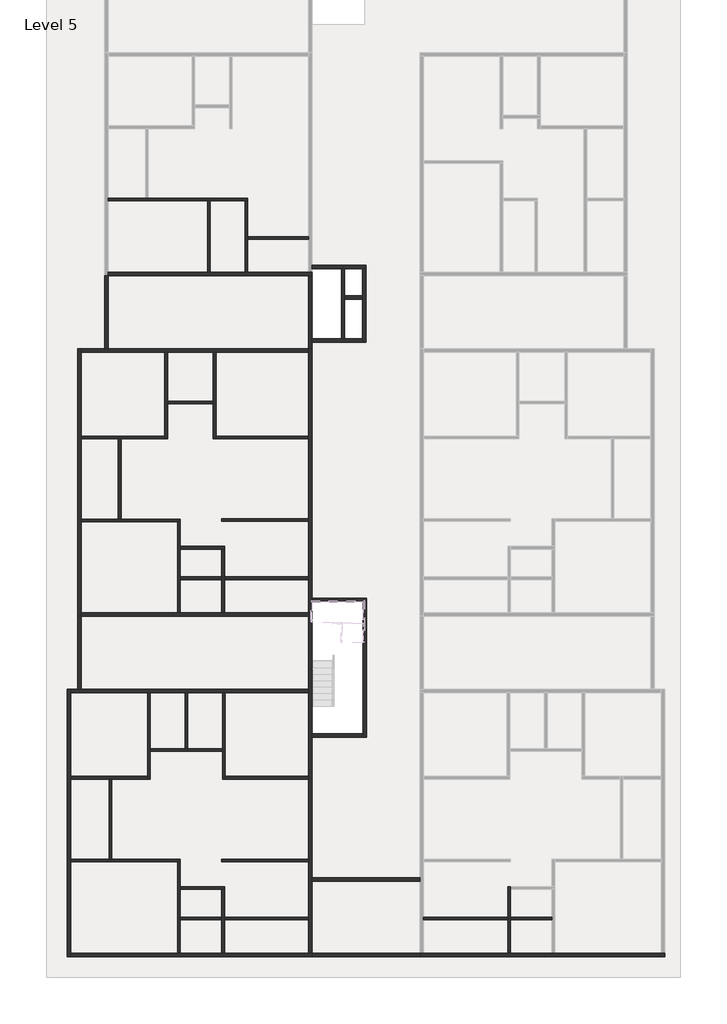
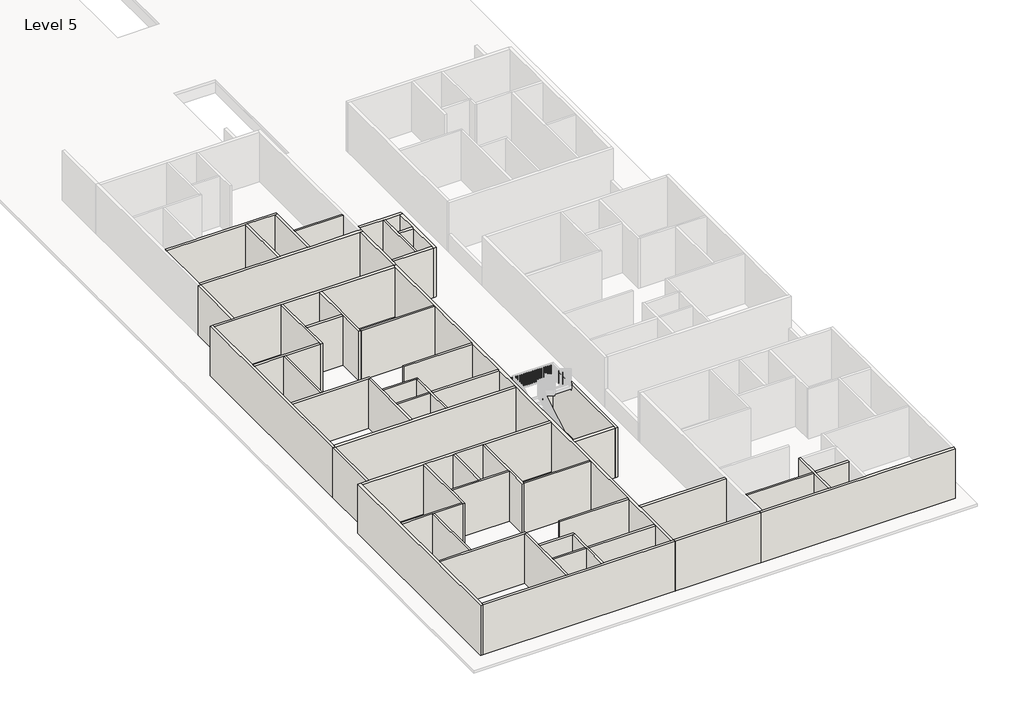
# One storey, part 1 of 8: 55 walls.
"""IFC4 building model written with IfcOpenShell, lengths in millimetres."""

from ifc_helpers import new_model, si_unit, frame, origin, place, context, project, spatial, polyline, outline, extrude, faceted_brep, element, save

model = new_model("IFC4")

# Units and contexts
model_context = context("Model", 3, world=origin())
ifc_project = project(units=[si_unit("LENGTHUNIT", "METRE", prefix="MILLI")], contexts=[model_context])

# Site, building, storey
site = spatial("IfcSite", under=ifc_project)
building = spatial("IfcBuilding", under=site)
storey = spatial("IfcBuildingStorey", under=building, Name="Level 5", Elevation=37426.6172466)

# Walls
placement = place(None, origin())
element("IfcWall", 1, ObjectType="4.5\"", at=placement, inside=storey, context=model_context, shape_type="Brep", body=[
    faceted_brep([(-12531.5544854, -1061.7344126, 37426.6172466), (-8188.1544854, -1061.7344126, 37426.6172466), (-8073.8544854, -1061.7344126, 37426.6172466), (-6549.8544854, -1061.7344126, 37426.6172466), (-6435.5544854, -1061.7344126, 37426.6172466), (-6435.5544854, -1061.7344126, 40474.6172466), (-6549.8544854, -1061.7344126, 40474.6172466), (-8073.8544854, -1061.7344126, 40474.6172466), (-8188.1544854, -1061.7344126, 40474.6172466), (-12531.5544854, -1061.7344126, 40474.6172466), (-12531.5544854, -947.4344126, 37426.6172466), (-12531.5544854, -947.4344126, 40474.6172466), (-10907.2415084, -947.4344126, 40474.6172466), (-10792.9415084, -947.4344126, 40474.6172466), (-6435.5544854, -947.4344126, 40474.6172466), (-6435.5544854, -947.4344126, 37426.6172466), (-10792.9415084, -947.4344126, 37426.6172466), (-10907.2415084, -947.4344126, 37426.6172466)], [[[0, 1, 2, 3, 4, 5, 6, 7, 8, 9]], [[10, 11, 12, 13, 14, 15, 16, 17]], [[4, 3, 2, 1, 0, 10, 17, 16, 15]], [[0, 9, 11, 10]], [[5, 4, 15, 14]], [[9, 8, 7, 6, 5, 14, 13, 12, 11]]]),
])
element("IfcWall", 2, ObjectType="4.5\"", at=placement, inside=storey, context=model_context, shape_type="Brep", body=[
    faceted_brep([(-6549.8544854, -1061.7344126, 37426.6172466), (-6549.8544854, -4185.9344126, 37426.6172466), (-6549.8544854, -4185.9344126, 40474.6172466), (-6549.8544854, -1061.7344126, 40474.6172466), (-6435.5544854, -1061.7344126, 37426.6172466), (-6435.5544854, -1061.7344126, 40474.6172466), (-6435.5544854, -2623.8344126, 40474.6172466), (-6435.5544854, -2738.1344126, 40474.6172466), (-6435.5544854, -4185.9344126, 40474.6172466), (-6435.5544854, -4185.9344126, 37426.6172466), (-6435.5544854, -2738.1344126, 37426.6172466), (-6435.5544854, -2623.8344126, 37426.6172466)], [[[0, 1, 2, 3]], [[4, 5, 6, 7, 8, 9, 10, 11]], [[1, 0, 4, 11, 10, 9]], [[0, 3, 5, 4]], [[2, 1, 9, 8]], [[3, 2, 8, 7, 6, 5]]]),
])
element("IfcWall", 3, ObjectType="4.5\"", at=placement, inside=storey, context=model_context, shape_type="SweptSolid", body=[
    extrude(outline(polyline([(-8188.1544854, -4185.9344126), (-8188.1544854, -1061.7344126), (-8073.8544854, -1061.7344126), (-8073.8544854, -4185.9344126), (-8188.1544854, -4185.9344126)])), frame((0.0, 0.0, 37426.6172466), z_axis=(0.0, 0.0, 1.0), x_axis=(1.0, 0.0, 0.0)), (0.0, 0.0, 1.0), 3048.0),
])
element("IfcWall", 4, ObjectType="4.5\"", at=placement, inside=storey, context=model_context, shape_type="SweptSolid", body=[
    extrude(outline(polyline([(-6435.5544854, -2623.8344126), (-3769.8415084, -2623.8344126), (-3769.8415084, -2738.1344126), (-6435.5544854, -2738.1344126), (-6435.5544854, -2623.8344126)])), frame((0.0, 0.0, 37426.6172466), z_axis=(0.0, 0.0, 1.0), x_axis=(1.0, 0.0, 0.0)), (0.0, 0.0, 1.0), 3048.0),
])
element("IfcWall", 5, ObjectType="4.5\"", at=placement, inside=storey, context=model_context, shape_type="Brep", body=[
    faceted_brep([(-10061.4044854, -7691.1344126, 37426.6172466), (-10061.4044854, -11348.7344126, 37426.6172466), (-10061.4044854, -11463.0344126, 37426.6172466), (-10061.4044854, -11463.0344126, 40474.6172466), (-10061.4044854, -11348.7344126, 40474.6172466), (-10061.4044854, -7691.1344126, 40474.6172466), (-9947.1044854, -7691.1344126, 37426.6172466), (-9947.1044854, -7691.1344126, 40474.6172466), (-9947.1044854, -9824.7344126, 40474.6172466), (-9947.1044854, -9939.0344126, 40474.6172466), (-9947.1044854, -11463.0344126, 40474.6172466), (-9947.1044854, -11463.0344126, 37426.6172466), (-9947.1044854, -9939.0344126, 37426.6172466), (-9947.1044854, -9824.7344126, 37426.6172466)], [[[0, 1, 2, 3, 4, 5]], [[6, 7, 8, 9, 10, 11, 12, 13]], [[2, 1, 0, 6, 13, 12, 11]], [[0, 5, 7, 6]], [[3, 2, 11, 10]], [[5, 4, 3, 10, 9, 8, 7]]]),
])
element("IfcWall", 6, ObjectType="4.5\"", at=placement, inside=storey, context=model_context, shape_type="Brep", body=[
    faceted_brep([(-10061.4044854, -11348.7344126, 37426.6172466), (-13719.0044854, -11348.7344126, 37426.6172466), (-13719.0044854, -11348.7344126, 40474.6172466), (-10061.4044854, -11348.7344126, 40474.6172466), (-10061.4044854, -11463.0344126, 37426.6172466), (-10061.4044854, -11463.0344126, 40474.6172466), (-11980.3915084, -11463.0344126, 40474.6172466), (-12094.6915084, -11463.0344126, 40474.6172466), (-13719.0044854, -11463.0344126, 40474.6172466), (-13719.0044854, -11463.0344126, 37426.6172466), (-12094.6915084, -11463.0344126, 37426.6172466), (-11980.3915084, -11463.0344126, 37426.6172466)], [[[0, 1, 2, 3]], [[4, 5, 6, 7, 8, 9, 10, 11]], [[1, 0, 4, 11, 10, 9]], [[0, 3, 5, 4]], [[2, 1, 9, 8]], [[3, 2, 8, 7, 6, 5]]]),
])
element("IfcWall", 7, ObjectType="4.5\"", at=placement, inside=storey, context=model_context, shape_type="SweptSolid", body=[
    extrude(outline(polyline([(-12094.6915084, -14968.2344126), (-12094.6915084, -11463.0344126), (-11980.3915084, -11463.0344126), (-11980.3915084, -14968.2344126), (-12094.6915084, -14968.2344126)])), frame((0.0, 0.0, 37426.6172466), z_axis=(0.0, 0.0, 1.0), x_axis=(1.0, 0.0, 0.0)), (0.0, 0.0, 1.0), 3048.0),
])
element("IfcWall", 8, ObjectType="4.5\"", at=placement, inside=storey, context=model_context, shape_type="Brep", body=[
    faceted_brep([(-13719.0044854, -15095.2344126, 37426.6172466), (-9510.2415084, -15095.2344126, 37426.6172466), (-9395.9415084, -15095.2344126, 37426.6172466), (-9395.9415084, -15095.2344126, 40474.6172466), (-9510.2415084, -15095.2344126, 40474.6172466), (-13719.0044854, -15095.2344126, 40474.6172466), (-13719.0044854, -14980.9344126, 37426.6172466), (-13719.0044854, -14980.9344126, 40474.6172466), (-9395.9415084, -14980.9344126, 40474.6172466), (-9395.9415084, -14980.9344126, 37426.6172466)], [[[0, 1, 2, 3, 4, 5]], [[6, 7, 8, 9]], [[2, 1, 0, 6, 9]], [[0, 5, 7, 6]], [[3, 2, 9, 8]], [[5, 4, 3, 8, 7]]]),
])
element("IfcWall", 9, ObjectType="4.5\"", at=placement, inside=storey, context=model_context, shape_type="Brep", body=[
    faceted_brep([(-9510.2415084, -15095.2344126, 37426.6172466), (-9510.2415084, -19070.3344126, 37426.6172466), (-9510.2415084, -19070.3344126, 40474.6172466), (-9510.2415084, -15095.2344126, 40474.6172466), (-9395.9415084, -15095.2344126, 37426.6172466), (-9395.9415084, -15095.2344126, 40474.6172466), (-9395.9415084, -16174.7344126, 40474.6172466), (-9395.9415084, -16289.0344126, 40474.6172466), (-9395.9415084, -17508.2344126, 40474.6172466), (-9395.9415084, -17622.5344126, 40474.6172466), (-9395.9415084, -19070.3344126, 40474.6172466), (-9395.9415084, -19070.3344126, 37426.6172466), (-9395.9415084, -17622.5344126, 37426.6172466), (-9395.9415084, -17508.2344126, 37426.6172466), (-9395.9415084, -16289.0344126, 37426.6172466), (-9395.9415084, -16174.7344126, 37426.6172466)], [[[0, 1, 2, 3]], [[4, 5, 6, 7, 8, 9, 10, 11, 12, 13, 14, 15]], [[1, 0, 4, 15, 14, 13, 12, 11]], [[0, 3, 5, 4]], [[2, 1, 11, 10]], [[3, 2, 10, 9, 8, 7, 6, 5]]]),
])
element("IfcWall", 10, ObjectType="4.5\"", at=placement, inside=storey, context=model_context, shape_type="Brep", body=[
    faceted_brep([(-9395.9415084, -16289.0344126, 37426.6172466), (-7567.1415084, -16289.0344126, 37426.6172466), (-7452.8415084, -16289.0344126, 37426.6172466), (-7452.8415084, -16289.0344126, 40474.6172466), (-7567.1415084, -16289.0344126, 40474.6172466), (-9395.9415084, -16289.0344126, 40474.6172466), (-9395.9415084, -16174.7344126, 37426.6172466), (-9395.9415084, -16174.7344126, 40474.6172466), (-7452.8415084, -16174.7344126, 40474.6172466), (-7452.8415084, -16174.7344126, 37426.6172466)], [[[0, 1, 2, 3, 4, 5]], [[6, 7, 8, 9]], [[2, 1, 0, 6, 9]], [[0, 5, 7, 6]], [[3, 2, 9, 8]], [[5, 4, 3, 8, 7]]]),
])
element("IfcWall", 11, ObjectType="4.5\"", at=placement, inside=storey, context=model_context, shape_type="Brep", body=[
    faceted_brep([(-7567.1415084, -16289.0344126, 37426.6172466), (-7567.1415084, -17508.2344126, 37426.6172466), (-7567.1415084, -17622.5344126, 37426.6172466), (-7567.1415084, -19070.3344126, 37426.6172466), (-7567.1415084, -19070.3344126, 40474.6172466), (-7567.1415084, -17622.5344126, 40474.6172466), (-7567.1415084, -17508.2344126, 40474.6172466), (-7567.1415084, -16289.0344126, 40474.6172466), (-7452.8415084, -16289.0344126, 37426.6172466), (-7452.8415084, -16289.0344126, 40474.6172466), (-7452.8415084, -17508.2344126, 40474.6172466), (-7452.8415084, -17622.5344126, 40474.6172466), (-7452.8415084, -19070.3344126, 40474.6172466), (-7452.8415084, -19070.3344126, 37426.6172466), (-7452.8415084, -17622.5344126, 37426.6172466), (-7452.8415084, -17508.2344126, 37426.6172466)], [[[0, 1, 2, 3, 4, 5, 6, 7]], [[8, 9, 10, 11, 12, 13, 14, 15]], [[3, 2, 1, 0, 8, 15, 14, 13]], [[0, 7, 9, 8]], [[4, 3, 13, 12]], [[7, 6, 5, 4, 12, 11, 10, 9]]]),
])
element("IfcWall", 12, ObjectType="4.5\"", at=placement, inside=storey, context=model_context, shape_type="SweptSolid", body=[
    extrude(outline(polyline([(-7567.1415084, -17622.5344126), (-9395.9415084, -17622.5344126), (-9395.9415084, -17508.2344126), (-7567.1415084, -17508.2344126), (-7567.1415084, -17622.5344126)])), frame((0.0, 0.0, 37426.6172466), z_axis=(0.0, 0.0, 1.0), x_axis=(1.0, 0.0, 0.0)), (0.0, 0.0, 1.0), 3048.0),
])
element("IfcWall", 13, ObjectType="4.5\"", at=placement, inside=storey, context=model_context, shape_type="SweptSolid", body=[
    extrude(outline(polyline([(-3769.8415084, -17622.5344126), (-7452.8415084, -17622.5344126), (-7452.8415084, -17508.2344126), (-3769.8415084, -17508.2344126), (-3769.8415084, -17622.5344126)])), frame((0.0, 0.0, 37426.6172466), z_axis=(0.0, 0.0, 1.0), x_axis=(1.0, 0.0, 0.0)), (0.0, 0.0, 1.0), 3048.0),
])
element("IfcWall", 14, ObjectType="4.5\"", at=placement, inside=storey, context=model_context, shape_type="SweptSolid", body=[
    extrude(outline(polyline([(-7567.1415084, -14968.2344126), (-3769.8415084, -14968.2344126), (-3769.8415084, -15082.5344126), (-7567.1415084, -15082.5344126), (-7567.1415084, -14968.2344126)])), frame((0.0, 0.0, 37426.6172466), z_axis=(0.0, 0.0, 1.0), x_axis=(1.0, 0.0, 0.0)), (0.0, 0.0, 1.0), 3048.0),
])
element("IfcWall", 15, ObjectType="4.5\"", at=placement, inside=storey, context=model_context, shape_type="SweptSolid", body=[
    extrude(outline(polyline([(-7940.5044854, -9939.0344126), (-9947.1044854, -9939.0344126), (-9947.1044854, -9824.7344126), (-7940.5044854, -9824.7344126), (-7940.5044854, -9939.0344126)])), frame((0.0, 0.0, 37426.6172466), z_axis=(0.0, 0.0, 1.0), x_axis=(1.0, 0.0, 0.0)), (0.0, 0.0, 1.0), 3048.0),
])
element("IfcWall", 16, ObjectType="4.5\"", at=placement, inside=storey, context=model_context, shape_type="Brep", body=[
    faceted_brep([(-7940.5044854, -7691.1344126, 37426.6172466), (-7940.5044854, -9824.7344126, 37426.6172466), (-7940.5044854, -9939.0344126, 37426.6172466), (-7940.5044854, -11463.0344126, 37426.6172466), (-7940.5044854, -11463.0344126, 40474.6172466), (-7940.5044854, -9939.0344126, 40474.6172466), (-7940.5044854, -9824.7344126, 40474.6172466), (-7940.5044854, -7691.1344126, 40474.6172466), (-7826.2044854, -7691.1344126, 37426.6172466), (-7826.2044854, -7691.1344126, 40474.6172466), (-7826.2044854, -11348.7344126, 40474.6172466), (-7826.2044854, -11463.0344126, 40474.6172466), (-7826.2044854, -11463.0344126, 37426.6172466), (-7826.2044854, -11348.7344126, 37426.6172466)], [[[0, 1, 2, 3, 4, 5, 6, 7]], [[8, 9, 10, 11, 12, 13]], [[3, 2, 1, 0, 8, 13, 12]], [[0, 7, 9, 8]], [[4, 3, 12, 11]], [[7, 6, 5, 4, 11, 10, 9]]]),
])
element("IfcWall", 17, ObjectType="4.5\"", at=placement, inside=storey, context=model_context, shape_type="SweptSolid", body=[
    extrude(outline(polyline([(-3769.8415084, -11463.0344126), (-7826.2044854, -11463.0344126), (-7826.2044854, -11348.7344126), (-3769.8415084, -11348.7344126), (-3769.8415084, -11463.0344126)])), frame((0.0, 0.0, 37426.6172466), z_axis=(0.0, 0.0, 1.0), x_axis=(1.0, 0.0, 0.0)), (0.0, 0.0, 1.0), 3048.0),
])
element("IfcWall", 18, ObjectType="4.5\"", at=placement, inside=storey, context=model_context, shape_type="Brep", body=[
    faceted_brep([(-10818.3415084, -22575.5344126, 37426.6172466), (-10818.3415084, -26233.1344126, 37426.6172466), (-10818.3415084, -26347.4344126, 37426.6172466), (-10818.3415084, -26347.4344126, 40474.6172466), (-10818.3415084, -26233.1344126, 40474.6172466), (-10818.3415084, -22575.5344126, 40474.6172466), (-10704.0415084, -22575.5344126, 37426.6172466), (-10704.0415084, -22575.5344126, 40474.6172466), (-10704.0415084, -25013.9344126, 40474.6172466), (-10704.0415084, -25128.2344126, 40474.6172466), (-10704.0415084, -26347.4344126, 40474.6172466), (-10704.0415084, -26347.4344126, 37426.6172466), (-10704.0415084, -25128.2344126, 37426.6172466), (-10704.0415084, -25013.9344126, 37426.6172466)], [[[0, 1, 2, 3, 4, 5]], [[6, 7, 8, 9, 10, 11, 12, 13]], [[2, 1, 0, 6, 13, 12, 11]], [[0, 5, 7, 6]], [[3, 2, 11, 10]], [[5, 4, 3, 10, 9, 8, 7]]]),
])
element("IfcWall", 19, ObjectType="4.5\"", at=placement, inside=storey, context=model_context, shape_type="Brep", body=[
    faceted_brep([(-10818.3415084, -26233.1344126, 37426.6172466), (-14171.1415084, -26233.1344126, 37426.6172466), (-14171.1415084, -26233.1344126, 40474.6172466), (-10818.3415084, -26233.1344126, 40474.6172466), (-10818.3415084, -26347.4344126, 37426.6172466), (-10818.3415084, -26347.4344126, 40474.6172466), (-12380.4415084, -26347.4344126, 40474.6172466), (-12494.7415084, -26347.4344126, 40474.6172466), (-14171.1415084, -26347.4344126, 40474.6172466), (-14171.1415084, -26347.4344126, 37426.6172466), (-12494.7415084, -26347.4344126, 37426.6172466), (-12380.4415084, -26347.4344126, 37426.6172466)], [[[0, 1, 2, 3]], [[4, 5, 6, 7, 8, 9, 10, 11]], [[1, 0, 4, 11, 10, 9]], [[0, 3, 5, 4]], [[2, 1, 9, 8]], [[3, 2, 8, 7, 6, 5]]]),
])
element("IfcWall", 20, ObjectType="4.5\"", at=placement, inside=storey, context=model_context, shape_type="SweptSolid", body=[
    extrude(outline(polyline([(-9180.0415084, -25013.9344126), (-9180.0415084, -22575.5344126), (-9065.7415084, -22575.5344126), (-9065.7415084, -25013.9344126), (-9180.0415084, -25013.9344126)])), frame((0.0, 0.0, 37426.6172466), z_axis=(0.0, 0.0, 1.0), x_axis=(1.0, 0.0, 0.0)), (0.0, 0.0, 1.0), 3048.0),
])
element("IfcWall", 21, ObjectType="4.5\"", at=placement, inside=storey, context=model_context, shape_type="Brep", body=[
    faceted_brep([(-10704.0415084, -25128.2344126, 37426.6172466), (-7541.7415084, -25128.2344126, 37426.6172466), (-7541.7415084, -25128.2344126, 40474.6172466), (-10704.0415084, -25128.2344126, 40474.6172466), (-10704.0415084, -25013.9344126, 37426.6172466), (-10704.0415084, -25013.9344126, 40474.6172466), (-9180.0415084, -25013.9344126, 40474.6172466), (-9065.7415084, -25013.9344126, 40474.6172466), (-7541.7415084, -25013.9344126, 40474.6172466), (-7541.7415084, -25013.9344126, 37426.6172466), (-9065.7415084, -25013.9344126, 37426.6172466), (-9180.0415084, -25013.9344126, 37426.6172466)], [[[0, 1, 2, 3]], [[4, 5, 6, 7, 8, 9, 10, 11]], [[1, 0, 4, 11, 10, 9]], [[0, 3, 5, 4]], [[2, 1, 9, 8]], [[3, 2, 8, 7, 6, 5]]]),
])
element("IfcWall", 22, ObjectType="4.5\"", at=placement, inside=storey, context=model_context, shape_type="Brep", body=[
    faceted_brep([(-7541.7415084, -22575.5344126, 37426.6172466), (-7541.7415084, -25013.9344126, 37426.6172466), (-7541.7415084, -25128.2344126, 37426.6172466), (-7541.7415084, -26347.4344126, 37426.6172466), (-7541.7415084, -26347.4344126, 40474.6172466), (-7541.7415084, -25128.2344126, 40474.6172466), (-7541.7415084, -25013.9344126, 40474.6172466), (-7541.7415084, -22575.5344126, 40474.6172466), (-7427.4415084, -22575.5344126, 37426.6172466), (-7427.4415084, -22575.5344126, 40474.6172466), (-7427.4415084, -26233.1344126, 40474.6172466), (-7427.4415084, -26347.4344126, 40474.6172466), (-7427.4415084, -26347.4344126, 37426.6172466), (-7427.4415084, -26233.1344126, 37426.6172466)], [[[0, 1, 2, 3, 4, 5, 6, 7]], [[8, 9, 10, 11, 12, 13]], [[3, 2, 1, 0, 8, 13, 12]], [[0, 7, 9, 8]], [[4, 3, 12, 11]], [[7, 6, 5, 4, 11, 10, 9]]]),
])
element("IfcWall", 23, ObjectType="4.5\"", at=placement, inside=storey, context=model_context, shape_type="SweptSolid", body=[
    extrude(outline(polyline([(-3769.8415084, -26347.4344126), (-7427.4415084, -26347.4344126), (-7427.4415084, -26233.1344126), (-3769.8415084, -26233.1344126), (-3769.8415084, -26347.4344126)])), frame((0.0, 0.0, 37426.6172466), z_axis=(0.0, 0.0, 1.0), x_axis=(1.0, 0.0, 0.0)), (0.0, 0.0, 1.0), 3048.0),
])
element("IfcWall", 24, ObjectType="4.5\"", at=placement, inside=storey, context=model_context, shape_type="SweptSolid", body=[
    extrude(outline(polyline([(-12494.7415084, -29852.6344126), (-12494.7415084, -26347.4344126), (-12380.4415084, -26347.4344126), (-12380.4415084, -29852.6344126), (-12494.7415084, -29852.6344126)])), frame((0.0, 0.0, 37426.6172466), z_axis=(0.0, 0.0, 1.0), x_axis=(1.0, 0.0, 0.0)), (0.0, 0.0, 1.0), 3048.0),
])
element("IfcWall", 25, ObjectType="4.5\"", at=placement, inside=storey, context=model_context, shape_type="Brep", body=[
    faceted_brep([(-14171.1415084, -29966.9344126, 37426.6172466), (-9510.2415084, -29966.9344126, 37426.6172466), (-9395.9415084, -29966.9344126, 37426.6172466), (-9395.9415084, -29966.9344126, 40474.6172466), (-9510.2415084, -29966.9344126, 40474.6172466), (-14171.1415084, -29966.9344126, 40474.6172466), (-14171.1415084, -29852.6344126, 37426.6172466), (-14171.1415084, -29852.6344126, 40474.6172466), (-12494.7415084, -29852.6344126, 40474.6172466), (-12380.4415084, -29852.6344126, 40474.6172466), (-9395.9415084, -29852.6344126, 40474.6172466), (-9395.9415084, -29852.6344126, 37426.6172466), (-12380.4415084, -29852.6344126, 37426.6172466), (-12494.7415084, -29852.6344126, 37426.6172466)], [[[0, 1, 2, 3, 4, 5]], [[6, 7, 8, 9, 10, 11, 12, 13]], [[2, 1, 0, 6, 13, 12, 11]], [[0, 5, 7, 6]], [[3, 2, 11, 10]], [[5, 4, 3, 10, 9, 8, 7]]]),
])
element("IfcWall", 26, ObjectType="4.5\"", at=placement, inside=storey, context=model_context, shape_type="Brep", body=[
    faceted_brep([(-9510.2415084, -29966.9344126, 37426.6172466), (-9510.2415084, -33954.7344126, 37426.6172466), (-9510.2415084, -33954.7344126, 40474.6172466), (-9510.2415084, -29966.9344126, 40474.6172466), (-9395.9415084, -29966.9344126, 37426.6172466), (-9395.9415084, -29966.9344126, 40474.6172466), (-9395.9415084, -31059.1344126, 40474.6172466), (-9395.9415084, -31173.4344126, 40474.6172466), (-9395.9415084, -32392.6344126, 40474.6172466), (-9395.9415084, -32506.9344126, 40474.6172466), (-9395.9415084, -33954.7344126, 40474.6172466), (-9395.9415084, -33954.7344126, 37426.6172466), (-9395.9415084, -32506.9344126, 37426.6172466), (-9395.9415084, -32392.6344126, 37426.6172466), (-9395.9415084, -31173.4344126, 37426.6172466), (-9395.9415084, -31059.1344126, 37426.6172466)], [[[0, 1, 2, 3]], [[4, 5, 6, 7, 8, 9, 10, 11, 12, 13, 14, 15]], [[1, 0, 4, 15, 14, 13, 12, 11]], [[0, 3, 5, 4]], [[2, 1, 11, 10]], [[3, 2, 10, 9, 8, 7, 6, 5]]]),
])
element("IfcWall", 27, ObjectType="4.5\"", at=placement, inside=storey, context=model_context, shape_type="Brep", body=[
    faceted_brep([(-9395.9415084, -31173.4344126, 37426.6172466), (-7567.1415084, -31173.4344126, 37426.6172466), (-7452.8415084, -31173.4344126, 37426.6172466), (-7452.8415084, -31173.4344126, 40474.6172466), (-7567.1415084, -31173.4344126, 40474.6172466), (-9395.9415084, -31173.4344126, 40474.6172466), (-9395.9415084, -31059.1344126, 37426.6172466), (-9395.9415084, -31059.1344126, 40474.6172466), (-7452.8415084, -31059.1344126, 40474.6172466), (-7452.8415084, -31059.1344126, 37426.6172466)], [[[0, 1, 2, 3, 4, 5]], [[6, 7, 8, 9]], [[2, 1, 0, 6, 9]], [[0, 5, 7, 6]], [[3, 2, 9, 8]], [[5, 4, 3, 8, 7]]]),
])
element("IfcWall", 28, ObjectType="4.5\"", at=placement, inside=storey, context=model_context, shape_type="Brep", body=[
    faceted_brep([(-7567.1415084, -31173.4344126, 37426.6172466), (-7567.1415084, -32392.6344126, 37426.6172466), (-7567.1415084, -32506.9344126, 37426.6172466), (-7567.1415084, -33954.7344126, 37426.6172466), (-7567.1415084, -33954.7344126, 40474.6172466), (-7567.1415084, -32506.9344126, 40474.6172466), (-7567.1415084, -32392.6344126, 40474.6172466), (-7567.1415084, -31173.4344126, 40474.6172466), (-7452.8415084, -31173.4344126, 37426.6172466), (-7452.8415084, -31173.4344126, 40474.6172466), (-7452.8415084, -32392.6344126, 40474.6172466), (-7452.8415084, -32506.9344126, 40474.6172466), (-7452.8415084, -33954.7344126, 40474.6172466), (-7452.8415084, -33954.7344126, 37426.6172466), (-7452.8415084, -32506.9344126, 37426.6172466), (-7452.8415084, -32392.6344126, 37426.6172466)], [[[0, 1, 2, 3, 4, 5, 6, 7]], [[8, 9, 10, 11, 12, 13, 14, 15]], [[3, 2, 1, 0, 8, 15, 14, 13]], [[0, 7, 9, 8]], [[4, 3, 13, 12]], [[7, 6, 5, 4, 12, 11, 10, 9]]]),
])
element("IfcWall", 29, ObjectType="4.5\"", at=placement, inside=storey, context=model_context, shape_type="SweptSolid", body=[
    extrude(outline(polyline([(-3769.8415084, -32392.6344126), (-3769.8415084, -32506.9344126), (-7452.8415084, -32506.9344126), (-7452.8415084, -32392.6344126), (-3769.8415084, -32392.6344126)])), frame((0.0, 0.0, 37426.6172466), z_axis=(0.0, 0.0, 1.0), x_axis=(1.0, 0.0, 0.0)), (0.0, 0.0, 1.0), 3048.0),
    extrude(outline(polyline([(-9395.9415084, -32506.9344126), (-9395.9415084, -32392.6344126), (-7567.1415084, -32392.6344126), (-7567.1415084, -32506.9344126), (-9395.9415084, -32506.9344126)])), frame((0.0, 0.0, 37426.6172466), z_axis=(0.0, 0.0, 1.0), x_axis=(1.0, 0.0, 0.0)), (0.0, 0.0, 1.0), 3048.0),
])
element("IfcWall", 30, ObjectType="4.5\"", at=placement, inside=storey, context=model_context, shape_type="SweptSolid", body=[
    extrude(outline(polyline([(-7567.1415084, -29852.6344126), (-3769.8415084, -29852.6344126), (-3769.8415084, -29966.9344126), (-7567.1415084, -29966.9344126), (-7567.1415084, -29852.6344126)])), frame((0.0, 0.0, 37426.6172466), z_axis=(0.0, 0.0, 1.0), x_axis=(1.0, 0.0, 0.0)), (0.0, 0.0, 1.0), 3048.0),
])
element("IfcWall", 31, ObjectType="4.5\"", at=placement, inside=storey, context=model_context, shape_type="SweptSolid", body=[
    extrude(outline(polyline([(4942.3584916, -32506.9344126), (1259.3584916, -32506.9344126), (1259.3584916, -32392.6344126), (4942.3584916, -32392.6344126), (4942.3584916, -32506.9344126)])), frame((0.0, 0.0, 37426.6172466), z_axis=(0.0, 0.0, 1.0), x_axis=(1.0, 0.0, 0.0)), (0.0, 0.0, 1.0), 3048.0),
])
element("IfcWall", 32, ObjectType="4.5\"", at=placement, inside=storey, context=model_context, shape_type="Brep", body=[
    faceted_brep([(4942.3584916, -31059.1344126, 37426.6172466), (4942.3584916, -32392.6344126, 37426.6172466), (4942.3584916, -32506.9344126, 37426.6172466), (4942.3584916, -33954.7344126, 37426.6172466), (4942.3584916, -33954.7344126, 40474.6172466), (4942.3584916, -32506.9344126, 40474.6172466), (4942.3584916, -32392.6344126, 40474.6172466), (4942.3584916, -31059.1344126, 40474.6172466), (5056.6584916, -31059.1344126, 37426.6172466), (5056.6584916, -31059.1344126, 40474.6172466), (5056.6584916, -31173.4344126, 40474.6172466), (5056.6584916, -32392.6344126, 40474.6172466), (5056.6584916, -32506.9344126, 40474.6172466), (5056.6584916, -33954.7344126, 40474.6172466), (5056.6584916, -33954.7344126, 37426.6172466), (5056.6584916, -32506.9344126, 37426.6172466), (5056.6584916, -32392.6344126, 37426.6172466), (5056.6584916, -31173.4344126, 37426.6172466)], [[[0, 1, 2, 3, 4, 5, 6, 7]], [[8, 9, 10, 11, 12, 13, 14, 15, 16, 17]], [[3, 2, 1, 0, 8, 17, 16, 15, 14]], [[4, 3, 14, 13]], [[0, 7, 9, 8]], [[7, 6, 5, 4, 13, 12, 11, 10, 9]]]),
])
element("IfcWall", 33, ObjectType="4.5\"", at=placement, inside=storey, context=model_context, shape_type="SweptSolid", body=[
    extrude(outline(polyline([(6885.4584916, -32506.9344126), (5056.6584916, -32506.9344126), (5056.6584916, -32392.6344126), (6885.4584916, -32392.6344126), (6885.4584916, -32506.9344126)])), frame((0.0, 0.0, 37426.6172466), z_axis=(0.0, 0.0, 1.0), x_axis=(1.0, 0.0, 0.0)), (0.0, 0.0, 1.0), 3048.0),
])
element("IfcWall", 34, ObjectType="4.5\"", at=placement, inside=storey, context=model_context, shape_type="Brep", body=[
    faceted_brep([(-2207.6738684, -7082.6751812, 37426.6172466), (-2207.6738684, -5366.3479894, 37426.6172466), (-2207.6738684, -5213.9479894, 37426.6172466), (-2207.6738684, -4034.6751812, 37426.6172466), (-2207.6738684, -4034.6751812, 40474.6172466), (-2207.6738684, -5213.9479894, 40474.6172466), (-2207.6738684, -5366.3479894, 40474.6172466), (-2207.6738684, -7082.6751812, 40474.6172466), (-2321.9738684, -7082.6751812, 37426.6172466), (-2321.9738684, -7082.6751812, 40474.6172466), (-2321.9738684, -4034.6751812, 40474.6172466), (-2321.9738684, -4034.6751812, 37426.6172466)], [[[0, 1, 2, 3, 4, 5, 6, 7]], [[8, 9, 10, 11]], [[3, 2, 1, 0, 8, 11]], [[7, 6, 5, 4, 10, 9]], [[4, 3, 11, 10]], [[0, 7, 9, 8]]]),
])
element("IfcWall", 35, ObjectType="6\"", at=placement, inside=storey, context=model_context, shape_type="Brep", body=[
    faceted_brep([(-12531.5544854, -4338.3344126, 37426.6172466), (-3769.8415084, -4338.3344126, 37426.6172466), (-3617.4415084, -4338.3344126, 37426.6172466), (-3617.4415084, -4338.3344126, 40474.6172466), (-3769.8415084, -4338.3344126, 40474.6172466), (-12531.5544854, -4338.3344126, 40474.6172466), (-12531.5544854, -4185.9344126, 37426.6172466), (-12531.5544854, -4185.9344126, 40474.6172466), (-8188.1544854, -4185.9344126, 40474.6172466), (-8073.8544854, -4185.9344126, 40474.6172466), (-6549.8544854, -4185.9344126, 40474.6172466), (-6435.5544854, -4185.9344126, 40474.6172466), (-3769.8415084, -4185.9344126, 40474.6172466), (-3617.4415084, -4185.9344126, 40474.6172466), (-3617.4415084, -4185.9344126, 37426.6172466), (-3769.8415084, -4185.9344126, 37426.6172466), (-6435.5544854, -4185.9344126, 37426.6172466), (-6549.8544854, -4185.9344126, 37426.6172466), (-8073.8544854, -4185.9344126, 37426.6172466), (-8188.1544854, -4185.9344126, 37426.6172466)], [[[0, 1, 2, 3, 4, 5]], [[6, 7, 8, 9, 10, 11, 12, 13, 14, 15, 16, 17, 18, 19]], [[2, 1, 0, 6, 19, 18, 17, 16, 15, 14]], [[0, 5, 7, 6]], [[3, 2, 14, 13]], [[5, 4, 3, 13, 12, 11, 10, 9, 8, 7]]]),
])
element("IfcWall", 36, ObjectType="6\"", at=placement, inside=storey, context=model_context, shape_type="Brep", body=[
    faceted_brep([(-13871.4044854, -7538.7344126, 37426.6172466), (-13871.4044854, -19222.7344126, 37426.6172466), (-13871.4044854, -19222.7344126, 40474.6172466), (-13871.4044854, -7538.7344126, 40474.6172466), (-13719.0044854, -7538.7344126, 37426.6172466), (-13719.0044854, -7538.7344126, 40474.6172466), (-13719.0044854, -7691.1344126, 40474.6172466), (-13719.0044854, -11348.7344126, 40474.6172466), (-13719.0044854, -11463.0344126, 40474.6172466), (-13719.0044854, -14980.9344126, 40474.6172466), (-13719.0044854, -15095.2344126, 40474.6172466), (-13719.0044854, -19070.3344126, 40474.6172466), (-13719.0044854, -19222.7344126, 40474.6172466), (-13719.0044854, -19222.7344126, 37426.6172466), (-13719.0044854, -19070.3344126, 37426.6172466), (-13719.0044854, -15095.2344126, 37426.6172466), (-13719.0044854, -14980.9344126, 37426.6172466), (-13719.0044854, -11463.0344126, 37426.6172466), (-13719.0044854, -11348.7344126, 37426.6172466), (-13719.0044854, -7691.1344126, 37426.6172466)], [[[0, 1, 2, 3]], [[4, 5, 6, 7, 8, 9, 10, 11, 12, 13, 14, 15, 16, 17, 18, 19]], [[1, 0, 4, 19, 18, 17, 16, 15, 14, 13]], [[2, 1, 13, 12]], [[0, 3, 5, 4]], [[3, 2, 12, 11, 10, 9, 8, 7, 6, 5]]]),
])
element("IfcWall", 37, ObjectType="6\"", at=placement, inside=storey, context=model_context, shape_type="Brep", body=[
    faceted_brep([(-13719.0044854, -19222.7344126, 37426.6172466), (-3769.8415084, -19222.7344126, 37426.6172466), (-3769.8415084, -19222.7344126, 40474.6172466), (-13719.0044854, -19222.7344126, 40474.6172466), (-13719.0044854, -19070.3344126, 37426.6172466), (-13719.0044854, -19070.3344126, 40474.6172466), (-9510.2415084, -19070.3344126, 40474.6172466), (-9395.9415084, -19070.3344126, 40474.6172466), (-7567.1415084, -19070.3344126, 40474.6172466), (-7452.8415084, -19070.3344126, 40474.6172466), (-3769.8415084, -19070.3344126, 40474.6172466), (-3769.8415084, -19070.3344126, 37426.6172466), (-7452.8415084, -19070.3344126, 37426.6172466), (-7567.1415084, -19070.3344126, 37426.6172466), (-9395.9415084, -19070.3344126, 37426.6172466), (-9510.2415084, -19070.3344126, 37426.6172466)], [[[0, 1, 2, 3]], [[4, 5, 6, 7, 8, 9, 10, 11, 12, 13, 14, 15]], [[1, 0, 4, 15, 14, 13, 12, 11]], [[0, 3, 5, 4]], [[2, 1, 11, 10]], [[3, 2, 10, 9, 8, 7, 6, 5]]]),
])
element("IfcWall", 38, ObjectType="6\"", at=placement, inside=storey, context=model_context, shape_type="Brep", body=[
    faceted_brep([(-3617.4415084, -33954.7344126, 37426.6172466), (-3617.4415084, -30820.9325185, 37426.6172466), (-3617.4415084, -30668.5325185, 37426.6172466), (-3617.4415084, -24525.9851539, 37426.6172466), (-3617.4415084, -24373.5851539, 37426.6172466), (-3617.4415084, -18582.3851539, 37426.6172466), (-3617.4415084, -18429.9851539, 37426.6172466), (-3617.4415084, -7538.7344126, 37426.6172466), (-3617.4415084, -7538.7344126, 40474.6172466), (-3617.4415084, -18429.9851539, 40474.6172466), (-3617.4415084, -18582.3851539, 40474.6172466), (-3617.4415084, -24373.5851539, 40474.6172466), (-3617.4415084, -24525.9851539, 40474.6172466), (-3617.4415084, -30668.5325185, 40474.6172466), (-3617.4415084, -30820.9325185, 40474.6172466), (-3617.4415084, -33954.7344126, 40474.6172466), (-3769.8415084, -33954.7344126, 37426.6172466), (-3769.8415084, -33954.7344126, 40474.6172466), (-3769.8415084, -32506.9344126, 40474.6172466), (-3769.8415084, -32392.6344126, 40474.6172466), (-3769.8415084, -29966.9344126, 40474.6172466), (-3769.8415084, -29852.6344126, 40474.6172466), (-3769.8415084, -26347.4344126, 40474.6172466), (-3769.8415084, -26233.1344126, 40474.6172466), (-3769.8415084, -22575.5344126, 40474.6172466), (-3769.8415084, -22423.1344126, 40474.6172466), (-3769.8415084, -19222.7344126, 40474.6172466), (-3769.8415084, -19070.3344126, 40474.6172466), (-3769.8415084, -17622.5344126, 40474.6172466), (-3769.8415084, -17508.2344126, 40474.6172466), (-3769.8415084, -15082.5344126, 40474.6172466), (-3769.8415084, -14968.2344126, 40474.6172466), (-3769.8415084, -11463.0344126, 40474.6172466), (-3769.8415084, -11348.7344126, 40474.6172466), (-3769.8415084, -7691.1344126, 40474.6172466), (-3769.8415084, -7538.7344126, 40474.6172466), (-3769.8415084, -7538.7344126, 37426.6172466), (-3769.8415084, -7691.1344126, 37426.6172466), (-3769.8415084, -11348.7344126, 37426.6172466), (-3769.8415084, -11463.0344126, 37426.6172466), (-3769.8415084, -14968.2344126, 37426.6172466), (-3769.8415084, -15082.5344126, 37426.6172466), (-3769.8415084, -17508.2344126, 37426.6172466), (-3769.8415084, -17622.5344126, 37426.6172466), (-3769.8415084, -19070.3344126, 37426.6172466), (-3769.8415084, -19222.7344126, 37426.6172466), (-3769.8415084, -22423.1344126, 37426.6172466), (-3769.8415084, -22575.5344126, 37426.6172466), (-3769.8415084, -26233.1344126, 37426.6172466), (-3769.8415084, -26347.4344126, 37426.6172466), (-3769.8415084, -29852.6344126, 37426.6172466), (-3769.8415084, -29966.9344126, 37426.6172466), (-3769.8415084, -32392.6344126, 37426.6172466), (-3769.8415084, -32506.9344126, 37426.6172466)], [[[0, 1, 2, 3, 4, 5, 6, 7, 8, 9, 10, 11, 12, 13, 14, 15]], [[16, 17, 18, 19, 20, 21, 22, 23, 24, 25, 26, 27, 28, 29, 30, 31, 32, 33, 34, 35, 36, 37, 38, 39, 40, 41, 42, 43, 44, 45, 46, 47, 48, 49, 50, 51, 52, 53]], [[7, 6, 5, 4, 3, 2, 1, 0, 16, 53, 52, 51, 50, 49, 48, 47, 46, 45, 44, 43, 42, 41, 40, 39, 38, 37, 36]], [[8, 7, 36, 35]], [[0, 15, 17, 16]], [[15, 14, 13, 12, 11, 10, 9, 8, 35, 34, 33, 32, 31, 30, 29, 28, 27, 26, 25, 24, 23, 22, 21, 20, 19, 18, 17]]]),
])
element("IfcWall", 39, ObjectType="6\"", at=placement, inside=storey, context=model_context, shape_type="Brep", body=[
    faceted_brep([(-3769.8415084, -7538.7344126, 37426.6172466), (-12531.5544854, -7538.7344126, 37426.6172466), (-12683.9544854, -7538.7344126, 37426.6172466), (-13719.0044854, -7538.7344126, 37426.6172466), (-13719.0044854, -7538.7344126, 40474.6172466), (-12683.9544854, -7538.7344126, 40474.6172466), (-12531.5544854, -7538.7344126, 40474.6172466), (-3769.8415084, -7538.7344126, 40474.6172466), (-3769.8415084, -7691.1344126, 37426.6172466), (-3769.8415084, -7691.1344126, 40474.6172466), (-7826.2044854, -7691.1344126, 40474.6172466), (-7940.5044854, -7691.1344126, 40474.6172466), (-9947.1044854, -7691.1344126, 40474.6172466), (-10061.4044854, -7691.1344126, 40474.6172466), (-13719.0044854, -7691.1344126, 40474.6172466), (-13719.0044854, -7691.1344126, 37426.6172466), (-10061.4044854, -7691.1344126, 37426.6172466), (-9947.1044854, -7691.1344126, 37426.6172466), (-7940.5044854, -7691.1344126, 37426.6172466), (-7826.2044854, -7691.1344126, 37426.6172466)], [[[0, 1, 2, 3, 4, 5, 6, 7]], [[8, 9, 10, 11, 12, 13, 14, 15, 16, 17, 18, 19]], [[3, 2, 1, 0, 8, 19, 18, 17, 16, 15]], [[0, 7, 9, 8]], [[4, 3, 15, 14]], [[7, 6, 5, 4, 14, 13, 12, 11, 10, 9]]]),
])
element("IfcWall", 40, ObjectType="6\"", at=placement, inside=storey, context=model_context, shape_type="Brep", body=[
    faceted_brep([(-14323.5415084, -22423.1344126, 37426.6172466), (-14323.5415084, -34107.1344126, 37426.6172466), (-14323.5415084, -34107.1344126, 40474.6172466), (-14323.5415084, -22423.1344126, 40474.6172466), (-14171.1415084, -22423.1344126, 37426.6172466), (-14171.1415084, -22423.1344126, 40474.6172466), (-14171.1415084, -22575.5344126, 40474.6172466), (-14171.1415084, -26233.1344126, 40474.6172466), (-14171.1415084, -26347.4344126, 40474.6172466), (-14171.1415084, -29852.6344126, 40474.6172466), (-14171.1415084, -29966.9344126, 40474.6172466), (-14171.1415084, -33954.7344126, 40474.6172466), (-14171.1415084, -34107.1344126, 40474.6172466), (-14171.1415084, -34107.1344126, 37426.6172466), (-14171.1415084, -33954.7344126, 37426.6172466), (-14171.1415084, -29966.9344126, 37426.6172466), (-14171.1415084, -29852.6344126, 37426.6172466), (-14171.1415084, -26347.4344126, 37426.6172466), (-14171.1415084, -26233.1344126, 37426.6172466), (-14171.1415084, -22575.5344126, 37426.6172466)], [[[0, 1, 2, 3]], [[4, 5, 6, 7, 8, 9, 10, 11, 12, 13, 14, 15, 16, 17, 18, 19]], [[1, 0, 4, 19, 18, 17, 16, 15, 14, 13]], [[2, 1, 13, 12]], [[0, 3, 5, 4]], [[3, 2, 12, 11, 10, 9, 8, 7, 6, 5]]]),
])
element("IfcWall", 41, ObjectType="6\"", at=placement, inside=storey, context=model_context, shape_type="Brep", body=[
    faceted_brep([(-14171.1415084, -34107.1344126, 37426.6172466), (-3617.4415084, -34107.1344126, 37426.6172466), (-3617.4415084, -34107.1344126, 40474.6172466), (-14171.1415084, -34107.1344126, 40474.6172466), (-14171.1415084, -33954.7344126, 37426.6172466), (-14171.1415084, -33954.7344126, 40474.6172466), (-9510.2415084, -33954.7344126, 40474.6172466), (-9395.9415084, -33954.7344126, 40474.6172466), (-7567.1415084, -33954.7344126, 40474.6172466), (-7452.8415084, -33954.7344126, 40474.6172466), (-3769.8415084, -33954.7344126, 40474.6172466), (-3617.4415084, -33954.7344126, 40474.6172466), (-3617.4415084, -33954.7344126, 37426.6172466), (-3769.8415084, -33954.7344126, 37426.6172466), (-7452.8415084, -33954.7344126, 37426.6172466), (-7567.1415084, -33954.7344126, 37426.6172466), (-9395.9415084, -33954.7344126, 37426.6172466), (-9510.2415084, -33954.7344126, 37426.6172466)], [[[0, 1, 2, 3]], [[4, 5, 6, 7, 8, 9, 10, 11, 12, 13, 14, 15, 16, 17]], [[1, 0, 4, 17, 16, 15, 14, 13, 12]], [[0, 3, 5, 4]], [[2, 1, 12, 11]], [[3, 2, 11, 10, 9, 8, 7, 6, 5]]]),
])
element("IfcWall", 42, ObjectType="6\"", at=placement, inside=storey, context=model_context, shape_type="Brep", body=[
    faceted_brep([(-3769.8415084, -22423.1344126, 37426.6172466), (-13719.0044854, -22423.1344126, 37426.6172466), (-13871.4044854, -22423.1344126, 37426.6172466), (-14171.1415084, -22423.1344126, 37426.6172466), (-14171.1415084, -22423.1344126, 40474.6172466), (-13871.4044854, -22423.1344126, 40474.6172466), (-13719.0044854, -22423.1344126, 40474.6172466), (-3769.8415084, -22423.1344126, 40474.6172466), (-3769.8415084, -22575.5344126, 37426.6172466), (-3769.8415084, -22575.5344126, 40474.6172466), (-7427.4415084, -22575.5344126, 40474.6172466), (-7541.7415084, -22575.5344126, 40474.6172466), (-9065.7415084, -22575.5344126, 40474.6172466), (-9180.0415084, -22575.5344126, 40474.6172466), (-10704.0415084, -22575.5344126, 40474.6172466), (-10818.3415084, -22575.5344126, 40474.6172466), (-14171.1415084, -22575.5344126, 40474.6172466), (-14171.1415084, -22575.5344126, 37426.6172466), (-10818.3415084, -22575.5344126, 37426.6172466), (-10704.0415084, -22575.5344126, 37426.6172466), (-9180.0415084, -22575.5344126, 37426.6172466), (-9065.7415084, -22575.5344126, 37426.6172466), (-7541.7415084, -22575.5344126, 37426.6172466), (-7427.4415084, -22575.5344126, 37426.6172466)], [[[0, 1, 2, 3, 4, 5, 6, 7]], [[8, 9, 10, 11, 12, 13, 14, 15, 16, 17, 18, 19, 20, 21, 22, 23]], [[3, 2, 1, 0, 8, 23, 22, 21, 20, 19, 18, 17]], [[0, 7, 9, 8]], [[4, 3, 17, 16]], [[7, 6, 5, 4, 16, 15, 14, 13, 12, 11, 10, 9]]]),
])
element("IfcWall", 43, ObjectType="6\"", at=placement, inside=storey, context=model_context, shape_type="Brep", body=[
    faceted_brep([(1106.9584916, -34107.1344126, 37426.6172466), (11813.0584916, -34107.1344126, 37426.6172466), (11813.0584916, -34107.1344126, 40474.6172466), (1106.9584916, -34107.1344126, 40474.6172466), (1106.9584916, -33954.7344126, 37426.6172466), (1106.9584916, -33954.7344126, 40474.6172466), (1259.3584916, -33954.7344126, 40474.6172466), (4942.3584916, -33954.7344126, 40474.6172466), (5056.6584916, -33954.7344126, 40474.6172466), (6885.4584916, -33954.7344126, 40474.6172466), (6999.7584916, -33954.7344126, 40474.6172466), (11660.6584916, -33954.7344126, 40474.6172466), (11813.0584916, -33954.7344126, 40474.6172466), (11813.0584916, -33954.7344126, 37426.6172466), (11660.6584916, -33954.7344126, 37426.6172466), (6999.7584916, -33954.7344126, 37426.6172466), (6885.4584916, -33954.7344126, 37426.6172466), (5056.6584916, -33954.7344126, 37426.6172466), (4942.3584916, -33954.7344126, 37426.6172466), (1259.3584916, -33954.7344126, 37426.6172466)], [[[0, 1, 2, 3]], [[4, 5, 6, 7, 8, 9, 10, 11, 12, 13, 14, 15, 16, 17, 18, 19]], [[1, 0, 4, 19, 18, 17, 16, 15, 14, 13]], [[2, 1, 13, 12]], [[0, 3, 5, 4]], [[3, 2, 12, 11, 10, 9, 8, 7, 6, 5]]]),
])
element("IfcWall", 44, ObjectType="6\"", at=placement, inside=storey, context=model_context, shape_type="Brep", body=[
    faceted_brep([(-3617.4415084, -18582.3851539, 37426.6172466), (-1382.2415084, -18582.3851539, 37426.6172466), (-1229.8415084, -18582.3851539, 37426.6172466), (-1229.8415084, -18582.3851539, 40474.6172466), (-1382.2415084, -18582.3851539, 40474.6172466), (-3617.4415084, -18582.3851539, 40474.6172466), (-3617.4415084, -18429.9851539, 37426.6172466), (-3617.4415084, -18429.9851539, 40474.6172466), (-1229.8415084, -18429.9851539, 40474.6172466), (-1229.8415084, -18429.9851539, 37426.6172466)], [[[0, 1, 2, 3, 4, 5]], [[6, 7, 8, 9]], [[2, 1, 0, 6, 9]], [[5, 4, 3, 8, 7]], [[0, 5, 7, 6]], [[3, 2, 9, 8]]]),
])
element("IfcWall", 45, ObjectType="6\"", at=placement, inside=storey, context=model_context, shape_type="Brep", body=[
    faceted_brep([(-1382.2415084, -18582.3851539, 37426.6172466), (-1382.2415084, -24373.5851539, 37426.6172466), (-1382.2415084, -24525.9851539, 37426.6172466), (-1382.2415084, -24525.9851539, 40474.6172466), (-1382.2415084, -24373.5851539, 40474.6172466), (-1382.2415084, -18582.3851539, 40474.6172466), (-1229.8415084, -18582.3851539, 37426.6172466), (-1229.8415084, -18582.3851539, 40474.6172466), (-1229.8415084, -24525.9851539, 40474.6172466), (-1229.8415084, -24525.9851539, 37426.6172466)], [[[0, 1, 2, 3, 4, 5]], [[6, 7, 8, 9]], [[2, 1, 0, 6, 9]], [[5, 4, 3, 8, 7]], [[0, 5, 7, 6]], [[3, 2, 9, 8]]]),
])
element("IfcWall", 46, ObjectType="6\"", at=placement, inside=storey, context=model_context, shape_type="SweptSolid", body=[
    extrude(outline(polyline([(-3617.4415084, -24373.5851539), (-1382.2415084, -24373.5851539), (-1382.2415084, -24525.9851539), (-3617.4415084, -24525.9851539), (-3617.4415084, -24373.5851539)])), frame((0.0, 0.0, 37426.6172466), z_axis=(0.0, 0.0, 1.0), x_axis=(1.0, 0.0, 0.0)), (0.0, 0.0, 1.0), 3048.0),
])
element("IfcWall", 47, ObjectType="6\"", at=placement, inside=storey, context=model_context, shape_type="Brep", body=[
    faceted_brep([(-3769.8415084, -4338.3344126, 37426.6172466), (-3769.8415084, -7538.7344126, 37426.6172466), (-3769.8415084, -7538.7344126, 40474.6172466), (-3769.8415084, -4338.3344126, 40474.6172466), (-3617.4415084, -4338.3344126, 37426.6172466), (-3617.4415084, -4338.3344126, 40474.6172466), (-3617.4415084, -7082.6751812, 40474.6172466), (-3617.4415084, -7235.0751812, 40474.6172466), (-3617.4415084, -7538.7344126, 40474.6172466), (-3617.4415084, -7538.7344126, 37426.6172466), (-3617.4415084, -7235.0751812, 37426.6172466), (-3617.4415084, -7082.6751812, 37426.6172466)], [[[0, 1, 2, 3]], [[4, 5, 6, 7, 8, 9, 10, 11]], [[1, 0, 4, 11, 10, 9]], [[0, 3, 5, 4]], [[2, 1, 9, 8]], [[3, 2, 8, 7, 6, 5]]]),
])
element("IfcWall", 48, ObjectType="6\"", at=placement, inside=storey, context=model_context, shape_type="Brep", body=[
    faceted_brep([(-3617.4415084, -4034.6751812, 37426.6172466), (-2321.9738684, -4034.6751812, 37426.6172466), (-2207.6738684, -4034.6751812, 37426.6172466), (-1407.6415084, -4034.6751812, 37426.6172466), (-1255.2415084, -4034.6751812, 37426.6172466), (-1255.2415084, -4034.6751812, 40474.6172466), (-1407.6415084, -4034.6751812, 40474.6172466), (-2207.6738684, -4034.6751812, 40474.6172466), (-2321.9738684, -4034.6751812, 40474.6172466), (-3617.4415084, -4034.6751812, 40474.6172466), (-3617.4415084, -3882.2751812, 37426.6172466), (-3617.4415084, -3882.2751812, 40474.6172466), (-1255.2415084, -3882.2751812, 40474.6172466), (-1255.2415084, -3882.2751812, 37426.6172466)], [[[0, 1, 2, 3, 4, 5, 6, 7, 8, 9]], [[10, 11, 12, 13]], [[4, 3, 2, 1, 0, 10, 13]], [[9, 8, 7, 6, 5, 12, 11]], [[0, 9, 11, 10]], [[5, 4, 13, 12]]]),
])
element("IfcWall", 49, ObjectType="6\"", at=placement, inside=storey, context=model_context, shape_type="Brep", body=[
    faceted_brep([(-1407.6415084, -4034.6751812, 37426.6172466), (-1407.6415084, -5213.9479894, 37426.6172466), (-1407.6415084, -5366.3479894, 37426.6172466), (-1407.6415084, -7082.6751812, 37426.6172466), (-1407.6415084, -7235.0751812, 37426.6172466), (-1407.6415084, -7235.0751812, 40474.6172466), (-1407.6415084, -7082.6751812, 40474.6172466), (-1407.6415084, -5366.3479894, 40474.6172466), (-1407.6415084, -5213.9479894, 40474.6172466), (-1407.6415084, -4034.6751812, 40474.6172466), (-1255.2415084, -4034.6751812, 37426.6172466), (-1255.2415084, -4034.6751812, 40474.6172466), (-1255.2415084, -7235.0751812, 40474.6172466), (-1255.2415084, -7235.0751812, 37426.6172466)], [[[0, 1, 2, 3, 4, 5, 6, 7, 8, 9]], [[10, 11, 12, 13]], [[4, 3, 2, 1, 0, 10, 13]], [[9, 8, 7, 6, 5, 12, 11]], [[0, 9, 11, 10]], [[5, 4, 13, 12]]]),
])
element("IfcWall", 50, ObjectType="6\"", at=placement, inside=storey, context=model_context, shape_type="Brep", body=[
    faceted_brep([(-1407.6415084, -7082.6751812, 37426.6172466), (-2207.6738684, -7082.6751812, 37426.6172466), (-2321.9738684, -7082.6751812, 37426.6172466), (-3617.4415084, -7082.6751812, 37426.6172466), (-3617.4415084, -7082.6751812, 40474.6172466), (-2321.9738684, -7082.6751812, 40474.6172466), (-2207.6738684, -7082.6751812, 40474.6172466), (-1407.6415084, -7082.6751812, 40474.6172466), (-1407.6415084, -7235.0751812, 37426.6172466), (-1407.6415084, -7235.0751812, 40474.6172466), (-3617.4415084, -7235.0751812, 40474.6172466), (-3617.4415084, -7235.0751812, 37426.6172466)], [[[0, 1, 2, 3, 4, 5, 6, 7]], [[8, 9, 10, 11]], [[3, 2, 1, 0, 8, 11]], [[7, 6, 5, 4, 10, 9]], [[0, 7, 9, 8]], [[4, 3, 11, 10]]]),
])
element("IfcWall", 51, ObjectType="6\"", at=placement, inside=storey, context=model_context, shape_type="SweptSolid", body=[
    extrude(outline(polyline([(-2207.6738684, -5213.9479894), (-1407.6415084, -5213.9479894), (-1407.6415084, -5366.3479894), (-2207.6738684, -5366.3479894), (-2207.6738684, -5213.9479894)])), frame((0.0, 0.0, 37426.6172466), z_axis=(0.0, 0.0, 1.0), x_axis=(1.0, 0.0, 0.0)), (0.0, 0.0, 1.0), 3048.0),
])
element("IfcWall", 52, ObjectType="6\" 2", at=placement, inside=storey, context=model_context, shape_type="SweptSolid", body=[
    extrude(outline(polyline([(1106.9584916, -34107.1344126), (-3617.4415084, -34107.1344126), (-3617.4415084, -33954.7344126), (1106.9584916, -33954.7344126), (1106.9584916, -34107.1344126)])), frame((0.0, 0.0, 37426.6172466), z_axis=(0.0, 0.0, 1.0), x_axis=(1.0, 0.0, 0.0)), (0.0, 0.0, 1.0), 3048.0),
])
element("IfcWall", 53, ObjectType="6\" 2", at=placement, inside=storey, context=model_context, shape_type="SweptSolid", body=[
    extrude(outline(polyline([(-3617.4415084, -30668.5325185), (1106.9584916, -30668.5325185), (1106.9584916, -30820.9325185), (-3617.4415084, -30820.9325185), (-3617.4415084, -30668.5325185)])), frame((0.0, 0.0, 37426.6172466), z_axis=(0.0, 0.0, 1.0), x_axis=(1.0, 0.0, 0.0)), (0.0, 0.0, 1.0), 3048.0),
])
element("IfcWall", 54, ObjectType="6\" 2", at=placement, inside=storey, context=model_context, shape_type="SweptSolid", body=[
    extrude(outline(polyline([(-13871.4044854, -22423.1344126), (-13871.4044854, -19222.7344126), (-13719.0044854, -19222.7344126), (-13719.0044854, -22423.1344126), (-13871.4044854, -22423.1344126)])), frame((0.0, 0.0, 37426.6172466), z_axis=(0.0, 0.0, 1.0), x_axis=(1.0, 0.0, 0.0)), (0.0, 0.0, 1.0), 3048.0),
])
element("IfcWall", 55, ObjectType="6\" 2", at=placement, inside=storey, context=model_context, shape_type="SweptSolid", body=[
    extrude(outline(polyline([(-12683.9544854, -7538.7344126), (-12683.9544854, -4338.3344126), (-12531.5544854, -4338.3344126), (-12531.5544854, -7538.7344126), (-12683.9544854, -7538.7344126)])), frame((0.0, 0.0, 37426.6172466), z_axis=(0.0, 0.0, 1.0), x_axis=(1.0, 0.0, 0.0)), (0.0, 0.0, 1.0), 3048.0),
])

save(model, "model.ifc")

# Revit data of these elements
# Type "4.5\""
#   Assembly Code = "B2010"
#   Layers, outside or top first: 0' - 4 1/2" "WALLS" (function 1)
# Type "6\""
#   Assembly Code = "B2010"
#   Layers, outside or top first: 0' - 6" "WALLS" (function 1)
# Type "6\" 2"
#   Assembly Code = "B2010"
#   Layers, outside or top first: 0' - 6" "4'" (function 1)
# Elements 1, 2, 3, 4, 5, 6, 7, 8, 9, 10, 11, 12, 13, 14, 15, 16, 17, 18, 19, 20, 21, 22, 23, 24, 25, 26, 27, 28, 29, 30, 31, 32, 33, 34 (IfcWall, "4.5\"")
#   Top Offset = 0' - 0"
#   Base Offset = 0' - 0"
#   Unconnected Height = 10' - 0"
#   wall height = 10' - 0"
#   Phase Created = New Construction
#   Base Constraint = Level 5
#   Materials on its faces: "WALLS"
# Elements 35, 36, 37, 38, 39, 40, 41, 42, 43, 44, 45, 46, 47, 48, 49, 50, 51 (IfcWall, "6\"")
#   Top Offset = 0' - 0"
#   Base Offset = 0' - 0"
#   Unconnected Height = 10' - 0"
#   wall height = 10' - 0"
#   Phase Created = New Construction
#   Base Constraint = Level 5
#   Materials on its faces: "WALLS"
# Elements 52, 53, 54, 55 (IfcWall, "6\" 2")
#   Top Offset = 0' - 0"
#   Base Offset = 0' - 0"
#   Unconnected Height = 10' - 0"
#   wall height = 10' - 0"
#   Phase Created = New Construction
#   Base Constraint = Level 5
#   Materials on its faces: "4'"
# Materials
#   "WALLS": class "Generic", colour RGB 120 120 120, transparency 0, Cost = 0
#   "4'": class "Generic", colour RGB 120 120 120, transparency 0, Cost = 0
